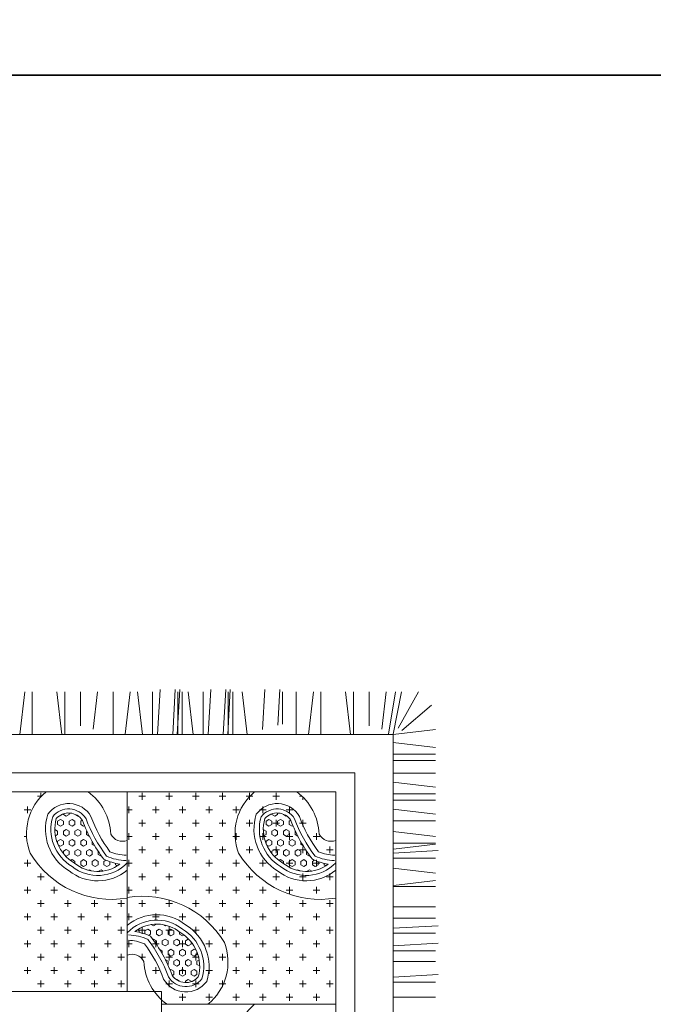
# Model space of a CAD drawing. Units: inches. Extents: x -638 to 186, y -762 to 59.
# Tile 19 of 31: x -118 to -92, y -243 to -203. Entities that reach past the tile are written whole.
import ezdxf

# ---------------------------------------------------------------- set-up
doc = ezdxf.new("R2010")
doc.units = ezdxf.units.IN
for name, color, linetype, lineweight in [('A-ANNO-DIMS', 2, 'Continuous', 18), ('furn', 8, 'Continuous', 13), ('wall', 7, 'Continuous', 35)]:
    doc.layers.add(name, color=color, linetype=linetype, lineweight=lineweight)
doc.styles.get("Standard").update_dxf_attribs({"font": 'arial.ttf'})
doc.dimstyles.new('ISO-25', dxfattribs={"dimtxt": 4, "dimasz": 4, "dimexe": 1.25, "dimexo": 0.625, "dimtad": 0, "dimlunit": 4, "dimtxsty": 'Standard', "dimcen": 2.5, "dimclrt": 256, "dimadec": 0, "dimazin": 0, "dimtfac": 1, "dimtmove": 0, "dimatfit": 3, "dimfxl": 1, "dimfxlon": 1, "dimarcsym": 0})

# ---------------------------------------------------------------- blocks, each defined once
blk = doc.blocks.new('BED-DOUBLE-WITH-NIGHTSTANDS')
for p, q in [((58.548, 11.244), (58.548, 59.951)), ((68.982, 31.914), (68.982, 1.829)), ((67.427, 30.359), (67.427, 3.384)), ((66.65, 29.582), (66.65, 4.161)), ((59.394, 16.552), (59.394, 16.825)), ((60.483, 16.552), (60.483, 16.825)), ((61.571, 16.552), (61.571, 16.825)), ((62.659, 16.552), (62.659, 16.825)), ((63.748, 16.552), (63.748, 16.825)), ((64.836, 16.726), (64.836, 16.825)), ((65.924, 16.552), (65.924, 16.825)), ((68.982, 17.003), (70.71, 16.797)), ((59.258, 16.688), (59.53, 16.688)), ((60.346, 16.688), (60.619, 16.688)), ((61.435, 16.688), (61.707, 16.688)), ((62.523, 16.688), (62.795, 16.688)), ((63.612, 16.688), (63.884, 16.688)), ((65.788, 16.688), (66.06, 16.688)), ((68.982, 16.497), (70.707, 16.497)), ((58.714, 16.144), (58.986, 16.144)), ((58.85, 16.008), (58.85, 16.28)), ((59.802, 16.144), (60.074, 16.144)), ((59.938, 16.008), (59.938, 16.28)), ((60.891, 16.144), (61.163, 16.144)), ((61.027, 16.008), (61.027, 16.28)), ((61.979, 16.144), (62.251, 16.144)), ((62.115, 16.008), (62.115, 16.28)), ((63.067, 16.144), (63.339, 16.144)), ((63.203, 16.008), (63.203, 16.28)), ((66.45, 16.144), (66.605, 16.144)), ((66.468, 16.127), (66.468, 16.28)), ((59.258, 15.6), (59.53, 15.6)), ((59.394, 15.464), (59.394, 15.736)), ((60.346, 15.6), (60.619, 15.6)), ((60.483, 15.464), (60.483, 15.736)), ((61.435, 15.6), (61.707, 15.6)), ((61.571, 15.464), (61.571, 15.736)), ((62.523, 15.6), (62.795, 15.6)), ((62.659, 15.464), (62.659, 15.736)), ((64.143, 15.233), (64.236, 15.233)), ((64.304, 15.115), (64.236, 15.233)), ((64.44, 15.351), (64.495, 15.445)), ((64.508, 15.233), (64.44, 15.351)), ((64.508, 15.233), (64.644, 15.233)), ((64.552, 15.469), (64.644, 15.469)), ((64.712, 15.351), (64.644, 15.469)), ((64.644, 15.233), (64.712, 15.351)), ((64.849, 15.115), (64.917, 15.233)), ((64.917, 15.469), (64.866, 15.556)), ((64.917, 15.469), (65.053, 15.469)), ((64.917, 15.233), (65.053, 15.233)), ((65.053, 15.469), (65.116, 15.579)), ((65.121, 15.115), (65.053, 15.233)), ((65.257, 15.351), (65.325, 15.469)), ((65.325, 15.233), (65.257, 15.351)), ((65.325, 15.469), (65.461, 15.469)), ((65.325, 15.233), (65.461, 15.233)), ((65.529, 15.351), (65.461, 15.469)), ((65.461, 15.233), (65.529, 15.351)), ((65.665, 15.115), (65.733, 15.233)), ((65.733, 15.233), (65.755, 15.233)), ((68.982, 15.294), (70.71, 15.497)), ((58.714, 15.056), (58.986, 15.056)), ((58.85, 14.92), (58.85, 15.192)), ((59.802, 15.056), (60.074, 15.056)), ((59.938, 14.92), (59.938, 15.192)), ((60.891, 15.056), (61.163, 15.056)), ((61.027, 14.92), (61.027, 15.192)), ((61.979, 15.056), (62.251, 15.056)), ((62.115, 14.92), (62.115, 15.192)), ((63.828, 14.762), (63.896, 14.88)), ((63.896, 14.88), (63.86, 14.942)), ((64.032, 15.115), (64.059, 15.161)), ((64.1, 14.997), (64.032, 15.115)), ((64.1, 14.997), (64.236, 14.997)), ((64.236, 14.997), (64.304, 15.115)), ((64.44, 14.88), (64.508, 14.997)), ((64.508, 14.762), (64.44, 14.88)), ((64.508, 14.997), (64.644, 14.997)), ((64.712, 14.88), (64.644, 14.997)), ((64.644, 14.762), (64.712, 14.88)), ((64.917, 14.997), (64.849, 15.115)), ((64.917, 14.997), (65.053, 14.997)), ((65.053, 14.997), (65.121, 15.115)), ((65.257, 14.88), (65.325, 14.997)), ((65.325, 14.762), (65.257, 14.88)), ((65.325, 14.997), (65.461, 14.997)), ((65.529, 14.88), (65.461, 14.997)), ((65.461, 14.762), (65.529, 14.88)), ((65.733, 14.997), (65.665, 15.115)), ((65.733, 14.997), (65.791, 14.997)), ((68.982, 15.174), (70.707, 15.174)), ((59.258, 14.512), (59.53, 14.512)), ((59.394, 14.376), (59.394, 14.648)), ((60.346, 14.512), (60.619, 14.512)), ((60.483, 14.376), (60.483, 14.648)), ((61.435, 14.512), (61.707, 14.512)), ((61.571, 14.376), (61.571, 14.648)), ((63.624, 14.408), (63.692, 14.526)), ((63.692, 14.291), (63.624, 14.408)), ((63.692, 14.526), (63.828, 14.526)), ((63.737, 14.762), (63.828, 14.762)), ((63.896, 14.408), (63.828, 14.526)), ((63.828, 14.291), (63.896, 14.408)), ((64.032, 14.644), (64.1, 14.762)), ((64.1, 14.526), (64.032, 14.644)), ((64.1, 14.762), (64.236, 14.762)), ((64.1, 14.526), (64.236, 14.526)), ((64.304, 14.644), (64.236, 14.762)), ((64.236, 14.526), (64.304, 14.644)), ((64.44, 14.408), (64.508, 14.526)), ((64.508, 14.291), (64.44, 14.408)), ((64.508, 14.762), (64.644, 14.762)), ((64.508, 14.526), (64.644, 14.526)), ((64.712, 14.408), (64.644, 14.526)), ((64.644, 14.291), (64.712, 14.408)), ((64.849, 14.644), (64.917, 14.762)), ((64.917, 14.526), (64.849, 14.644)), ((64.917, 14.762), (65.053, 14.762)), ((64.917, 14.526), (65.053, 14.526)), ((65.121, 14.644), (65.053, 14.762)), ((65.053, 14.526), (65.121, 14.644)), ((65.257, 14.408), (65.325, 14.526)), ((65.276, 14.375), (65.257, 14.408)), ((65.325, 14.762), (65.461, 14.762)), ((65.325, 14.526), (65.461, 14.526)), ((65.497, 14.464), (65.461, 14.526)), ((65.665, 14.644), (65.733, 14.762)), ((65.671, 14.634), (65.665, 14.644)), ((65.733, 14.762), (65.741, 14.762)), ((69.331, 14.538), (70.707, 14.538)), ((58.85, 13.832), (58.85, 14.104)), ((59.938, 13.832), (59.938, 14.104)), ((61.027, 13.832), (61.027, 14.104)), ((62.115, 13.832), (62.115, 14.104)), ((63.438, 14.086), (63.488, 14.173)), ((63.488, 14.173), (63.465, 14.213)), ((63.624, 13.937), (63.692, 14.055)), ((63.692, 14.291), (63.828, 14.291)), ((63.692, 14.055), (63.828, 14.055)), ((63.896, 13.937), (63.828, 14.055)), ((64.032, 14.173), (64.1, 14.291)), ((64.1, 14.055), (64.032, 14.173)), ((64.1, 14.291), (64.236, 14.291)), ((64.1, 14.055), (64.236, 14.055)), ((64.304, 14.173), (64.236, 14.291)), ((64.236, 14.055), (64.304, 14.173)), ((64.451, 13.955), (64.508, 14.055)), ((64.508, 14.291), (64.644, 14.291)), ((64.508, 14.055), (64.621, 14.055)), ((64.852, 14.179), (64.917, 14.291)), ((64.917, 14.291), (65.053, 14.291)), ((65.059, 14.28), (65.053, 14.291)), ((69.195, 14.023), (70.71, 13.844)), ((58.714, 13.968), (58.986, 13.968)), ((59.802, 13.968), (60.074, 13.968)), ((60.891, 13.968), (61.163, 13.968)), ((61.979, 13.968), (62.251, 13.968)), ((63.417, 13.819), (63.42, 13.819)), ((63.488, 13.701), (63.42, 13.819)), ((63.434, 13.608), (63.488, 13.701)), ((63.692, 13.819), (63.624, 13.937)), ((63.692, 13.819), (63.828, 13.819)), ((63.828, 13.819), (63.896, 13.937)), ((64.032, 13.701), (64.1, 13.819)), ((64.043, 13.682), (64.032, 13.701)), ((64.1, 13.819), (64.236, 13.819)), ((64.237, 13.818), (64.236, 13.819)), ((59.258, 13.423), (59.53, 13.423)), ((59.394, 13.287), (59.394, 13.559)), ((60.346, 13.423), (60.619, 13.423)), ((60.483, 13.287), (60.483, 13.559)), ((61.435, 13.423), (61.707, 13.423)), ((61.571, 13.287), (61.571, 13.559)), ((63.624, 13.466), (63.692, 13.584)), ((63.692, 13.348), (63.624, 13.466)), ((63.692, 13.584), (63.828, 13.584)), ((63.692, 13.348), (63.815, 13.348)), ((63.874, 13.504), (63.828, 13.584)), ((68.996, 13.214), (70.707, 13.214)), ((58.714, 12.879), (58.986, 12.879)), ((58.85, 12.743), (58.85, 13.015)), ((59.802, 12.879), (60.074, 12.879)), ((59.938, 12.743), (59.938, 13.015)), ((60.891, 12.879), (61.163, 12.879)), ((61.027, 12.743), (61.027, 13.015)), ((61.979, 12.879), (62.251, 12.879)), ((62.115, 12.743), (62.115, 13.015)), ((63.648, 13.036), (63.692, 13.112)), ((63.692, 13.112), (63.748, 13.112)), ((66.65, 12.635), (58.548, 12.635)), ((58.548, 12.635), (66.65, 12.635)), ((60.346, 12.568), (60.619, 12.568)), ((60.483, 12.432), (60.483, 12.635)), ((61.435, 12.568), (61.707, 12.568)), ((61.571, 12.432), (61.571, 12.635)), ((62.523, 12.568), (62.795, 12.568)), ((62.523, 12.568), (62.795, 12.568)), ((62.659, 12.432), (62.659, 12.635)), ((62.659, 12.432), (62.659, 12.635)), ((63.612, 12.568), (63.884, 12.568)), ((63.612, 12.568), (63.884, 12.568)), ((63.748, 12.432), (63.748, 12.635)), ((63.748, 12.432), (63.748, 12.635)), ((64.7, 12.568), (64.972, 12.568)), ((64.7, 12.568), (64.972, 12.568)), ((64.836, 12.432), (64.836, 12.635)), ((64.836, 12.432), (64.836, 12.635)), ((65.788, 12.568), (66.06, 12.568)), ((65.788, 12.568), (66.06, 12.568)), ((65.924, 12.432), (65.924, 12.635)), ((65.924, 12.432), (65.924, 12.635)), ((66.65, 12.635), (66.65, 4.161)), ((68.996, 12.723), (70.71, 12.52)), ((59.857, 12.024), (60.074, 12.024)), ((59.938, 11.888), (59.938, 12.107)), ((60.891, 12.024), (61.163, 12.024)), ((61.003, 12.157), (60.948, 12.157)), ((61.047, 12.233), (61.003, 12.157)), ((61.027, 11.888), (61.027, 12.16)), ((61.979, 12.024), (62.251, 12.024)), ((62.115, 11.888), (62.115, 12.16)), ((63.067, 12.024), (63.339, 12.024)), ((63.067, 12.024), (63.339, 12.024)), ((63.203, 11.888), (63.203, 12.16)), ((63.203, 11.888), (63.203, 12.16)), ((64.156, 12.024), (64.428, 12.024)), ((64.156, 12.024), (64.428, 12.024)), ((64.292, 11.888), (64.292, 12.16)), ((64.292, 11.888), (64.292, 12.16)), ((65.244, 12.024), (65.516, 12.024)), ((65.244, 12.024), (65.516, 12.024)), ((65.38, 11.888), (65.38, 12.16)), ((65.38, 11.888), (65.38, 12.16)), ((66.332, 12.024), (66.605, 12.024)), ((66.332, 12.024), (66.605, 12.024)), ((66.468, 11.888), (66.468, 12.16)), ((66.468, 11.888), (66.468, 12.16)), ((68.982, 12.011), (70.71, 12.214)), ((59.394, 11.344), (59.394, 11.616)), ((60.483, 11.344), (60.483, 11.616)), ((60.821, 11.766), (60.867, 11.686)), ((61.003, 11.686), (60.867, 11.686)), ((61.003, 11.921), (60.881, 11.921)), ((61.003, 11.921), (61.072, 11.804)), ((61.072, 11.804), (61.003, 11.686)), ((61.261, 11.661), (61.208, 11.568)), ((61.571, 11.344), (61.571, 11.616)), ((62.659, 11.344), (62.659, 11.616)), ((62.659, 11.344), (62.659, 11.616)), ((63.748, 11.344), (63.748, 11.616)), ((63.748, 11.344), (63.748, 11.616)), ((64.836, 11.344), (64.836, 11.616)), ((64.836, 11.344), (64.836, 11.616)), ((65.924, 11.344), (65.924, 11.616)), ((65.924, 11.344), (65.924, 11.616)), ((68.982, 11.603), (70.71, 11.603)), ((20.158, 11.244), (58.548, 11.244)), ((58.022, 4.161), (58.022, 11.244)), ((58.022, 11.244), (58.022, 4.161)), ((59.258, 11.48), (59.53, 11.48)), ((60.187, 11.215), (60.075, 11.215)), ((60.245, 11.315), (60.187, 11.215)), ((60.346, 11.48), (60.619, 11.48)), ((60.459, 11.215), (60.391, 11.097)), ((60.459, 11.451), (60.459, 11.45)), ((60.595, 11.45), (60.459, 11.45)), ((60.595, 11.215), (60.459, 11.215)), ((60.663, 11.568), (60.595, 11.45)), ((60.595, 11.215), (60.663, 11.097)), ((60.652, 11.587), (60.663, 11.568)), ((60.867, 11.45), (60.799, 11.332)), ((60.799, 11.332), (60.867, 11.215)), ((61.003, 11.45), (60.867, 11.45)), ((61.003, 11.215), (60.867, 11.215)), ((61.003, 11.45), (61.072, 11.332)), ((61.072, 11.332), (61.003, 11.215)), ((61.208, 11.568), (61.276, 11.45)), ((61.279, 11.45), (61.276, 11.45)), ((61.435, 11.48), (61.707, 11.48)), ((62.523, 11.48), (62.795, 11.48)), ((62.523, 11.48), (62.795, 11.48)), ((63.612, 11.48), (63.884, 11.48)), ((63.612, 11.48), (63.884, 11.48)), ((64.7, 11.48), (64.972, 11.48)), ((64.7, 11.48), (64.972, 11.48)), ((65.788, 11.48), (66.06, 11.48)), ((65.788, 11.48), (66.06, 11.48)), ((68.982, 11.4), (70.811, 11.298)), ((58.714, 10.936), (58.986, 10.936)), ((58.85, 10.8), (58.85, 11.072)), ((59.199, 10.806), (59.235, 10.743)), ((59.439, 10.861), (59.371, 10.743)), ((59.419, 10.895), (59.439, 10.861)), ((59.637, 10.99), (59.643, 10.979)), ((59.779, 10.979), (59.643, 10.979)), ((59.843, 11.09), (59.779, 10.979)), ((59.802, 10.936), (60.074, 10.936)), ((59.938, 10.8), (59.938, 11.072)), ((60.051, 10.979), (59.983, 10.861)), ((59.983, 10.861), (60.051, 10.743)), ((60.187, 10.979), (60.051, 10.979)), ((60.187, 10.979), (60.255, 10.861)), ((60.255, 10.861), (60.187, 10.743)), ((60.391, 11.097), (60.459, 10.979)), ((60.595, 10.979), (60.459, 10.979)), ((60.663, 11.097), (60.595, 10.979)), ((60.867, 10.979), (60.799, 10.861)), ((60.799, 10.861), (60.867, 10.743)), ((61.003, 10.979), (60.867, 10.979)), ((60.891, 10.936), (61.163, 10.936)), ((61.003, 10.979), (61.072, 10.861)), ((61.072, 10.861), (61.003, 10.743)), ((61.027, 10.8), (61.027, 11.072)), ((61.258, 11.184), (61.208, 11.097)), ((61.208, 11.097), (61.231, 11.057)), ((61.979, 10.936), (62.251, 10.936)), ((62.115, 10.8), (62.115, 11.072)), ((63.067, 10.936), (63.339, 10.936)), ((63.067, 10.936), (63.339, 10.936)), ((63.203, 10.8), (63.203, 11.072)), ((63.203, 10.8), (63.203, 11.072)), ((64.156, 10.936), (64.428, 10.936)), ((64.156, 10.936), (64.428, 10.936)), ((64.292, 10.8), (64.292, 11.072)), ((64.292, 10.8), (64.292, 11.072)), ((65.244, 10.936), (65.516, 10.936)), ((65.244, 10.936), (65.516, 10.936)), ((65.38, 10.8), (65.38, 11.072)), ((65.38, 10.8), (65.38, 11.072)), ((66.332, 10.936), (66.605, 10.936)), ((66.332, 10.936), (66.605, 10.936)), ((66.468, 10.8), (66.468, 11.072)), ((66.468, 10.8), (66.468, 11.072)), ((58.306, 10.256), (58.306, 10.528)), ((58.963, 10.508), (58.955, 10.508)), ((59.031, 10.625), (58.963, 10.508)), ((59.025, 10.636), (59.031, 10.625)), ((59.235, 10.508), (59.167, 10.39)), ((59.371, 10.743), (59.235, 10.743)), ((59.371, 10.508), (59.235, 10.508)), ((59.371, 10.508), (59.439, 10.39)), ((59.394, 10.256), (59.394, 10.528)), ((59.643, 10.743), (59.575, 10.625)), ((59.575, 10.625), (59.643, 10.508)), ((59.779, 10.743), (59.643, 10.743)), ((59.779, 10.508), (59.643, 10.508)), ((59.779, 10.743), (59.847, 10.625)), ((59.847, 10.625), (59.779, 10.508)), ((60.051, 10.508), (59.983, 10.39)), ((60.187, 10.743), (60.051, 10.743)), ((60.187, 10.508), (60.051, 10.508)), ((60.187, 10.508), (60.255, 10.39)), ((60.459, 10.743), (60.391, 10.625)), ((60.391, 10.625), (60.459, 10.508)), ((60.595, 10.743), (60.459, 10.743)), ((60.595, 10.508), (60.459, 10.508)), ((60.483, 10.256), (60.483, 10.528)), ((60.595, 10.743), (60.663, 10.625)), ((60.663, 10.625), (60.595, 10.508)), ((60.867, 10.508), (60.799, 10.39)), ((61.003, 10.743), (60.867, 10.743)), ((60.958, 10.508), (60.867, 10.508)), ((61.571, 10.256), (61.571, 10.528)), ((62.659, 10.256), (62.659, 10.528)), ((62.659, 10.256), (62.659, 10.528)), ((63.748, 10.256), (63.748, 10.528)), ((63.748, 10.256), (63.748, 10.528)), ((64.836, 10.256), (64.836, 10.528)), ((64.836, 10.256), (64.836, 10.528)), ((65.924, 10.256), (65.924, 10.528)), ((65.924, 10.256), (65.924, 10.528)), ((68.982, 10.789), (70.811, 10.687)), ((68.982, 10.606), (70.811, 10.504)), ((68.982, 10.585), (70.71, 10.585)), ((68.982, 10.402), (70.71, 10.402)), ((58.17, 10.392), (58.442, 10.392)), ((58.963, 10.272), (58.904, 10.272)), ((58.963, 10.036), (58.94, 10.036)), ((58.963, 10.272), (59.031, 10.154)), ((59.031, 10.154), (58.963, 10.036)), ((59.167, 10.39), (59.235, 10.272)), ((59.235, 10.036), (59.167, 9.919)), ((59.371, 10.272), (59.235, 10.272)), ((59.371, 10.036), (59.235, 10.036)), ((59.258, 10.392), (59.53, 10.392)), ((59.439, 10.39), (59.371, 10.272)), ((59.371, 10.036), (59.439, 9.919)), ((59.643, 10.272), (59.575, 10.154)), ((59.575, 10.154), (59.643, 10.036)), ((59.779, 10.272), (59.643, 10.272)), ((59.779, 10.036), (59.643, 10.036)), ((59.779, 10.272), (59.847, 10.154)), ((59.847, 10.154), (59.779, 10.036)), ((59.983, 10.39), (60.051, 10.272)), ((60.051, 10.036), (59.983, 9.919)), ((60.187, 10.272), (60.051, 10.272)), ((60.187, 10.036), (60.051, 10.036)), ((60.255, 10.39), (60.187, 10.272)), ((60.187, 10.036), (60.255, 9.919)), ((60.346, 10.392), (60.619, 10.392)), ((60.459, 10.272), (60.391, 10.154)), ((60.391, 10.154), (60.459, 10.036)), ((60.595, 10.272), (60.459, 10.272)), ((60.553, 10.036), (60.459, 10.036)), ((60.595, 10.272), (60.663, 10.154)), ((60.663, 10.154), (60.637, 10.108)), ((60.799, 10.39), (60.836, 10.327)), ((61.435, 10.392), (61.707, 10.392)), ((62.523, 10.392), (62.795, 10.392)), ((62.523, 10.392), (62.795, 10.392)), ((63.612, 10.392), (63.884, 10.392)), ((63.612, 10.392), (63.884, 10.392)), ((64.7, 10.392), (64.972, 10.392)), ((64.7, 10.392), (64.972, 10.392)), ((65.788, 10.392), (66.06, 10.392)), ((65.788, 10.392), (66.06, 10.392)), ((68.982, 9.957), (70.71, 10.161)), ((58.714, 9.847), (58.986, 9.847)), ((58.85, 9.711), (58.85, 9.983)), ((59.167, 9.919), (59.235, 9.801)), ((59.371, 9.801), (59.235, 9.801)), ((59.439, 9.919), (59.371, 9.801)), ((59.643, 9.801), (59.58, 9.691)), ((59.779, 9.801), (59.643, 9.801)), ((59.779, 9.801), (59.83, 9.713)), ((59.802, 9.847), (60.074, 9.847)), ((59.938, 9.711), (59.938, 9.983)), ((59.983, 9.919), (60.051, 9.801)), ((60.144, 9.801), (60.051, 9.801)), ((60.255, 9.919), (60.201, 9.825)), ((60.891, 9.847), (61.163, 9.847)), ((61.027, 9.711), (61.027, 9.983)), ((61.979, 9.847), (62.251, 9.847)), ((61.979, 9.847), (62.251, 9.847)), ((62.115, 9.711), (62.115, 9.983)), ((62.115, 9.711), (62.115, 9.983)), ((63.067, 9.847), (63.339, 9.847)), ((63.067, 9.847), (63.339, 9.847)), ((63.203, 9.711), (63.203, 9.983)), ((63.203, 9.711), (63.203, 9.983)), ((64.156, 9.847), (64.428, 9.847)), ((64.156, 9.847), (64.428, 9.847)), ((64.292, 9.711), (64.292, 9.983)), ((64.292, 9.711), (64.292, 9.983)), ((65.244, 9.847), (65.516, 9.847)), ((65.244, 9.847), (65.516, 9.847)), ((65.38, 9.711), (65.38, 9.983)), ((65.38, 9.711), (65.38, 9.983)), ((66.332, 9.847), (66.605, 9.847)), ((66.332, 9.847), (66.605, 9.847)), ((66.468, 9.711), (66.468, 9.983)), ((66.468, 9.711), (66.468, 9.983)), ((58.17, 9.303), (58.442, 9.303)), ((58.306, 9.167), (58.306, 9.439)), ((59.258, 9.303), (59.53, 9.303)), ((59.394, 9.167), (59.394, 9.439)), ((60.346, 9.303), (60.619, 9.303)), ((60.483, 9.167), (60.483, 9.439)), ((61.435, 9.303), (61.707, 9.303)), ((61.435, 9.303), (61.707, 9.303)), ((61.571, 9.167), (61.571, 9.439)), ((61.571, 9.167), (61.571, 9.439)), ((62.523, 9.303), (62.795, 9.303)), ((62.523, 9.303), (62.795, 9.303)), ((62.659, 9.167), (62.659, 9.439)), ((62.659, 9.167), (62.659, 9.439)), ((63.612, 9.303), (63.884, 9.303)), ((63.612, 9.303), (63.884, 9.303)), ((63.748, 9.167), (63.748, 9.439)), ((63.748, 9.167), (63.748, 9.439)), ((64.7, 9.303), (64.972, 9.303)), ((64.7, 9.303), (64.972, 9.303)), ((64.836, 9.167), (64.836, 9.439)), ((64.836, 9.167), (64.836, 9.439)), ((65.788, 9.303), (66.06, 9.303)), ((65.788, 9.303), (66.06, 9.303)), ((65.924, 9.167), (65.924, 9.439)), ((65.924, 9.167), (65.924, 9.439)), ((68.982, 9.55), (70.71, 9.55)), ((68.982, 9.347), (70.811, 9.245)), ((58.85, 8.623), (58.85, 8.895)), ((59.938, 8.623), (59.938, 8.895)), ((61.027, 8.623), (61.027, 8.895)), ((61.027, 8.623), (61.027, 8.895)), ((62.115, 8.623), (62.115, 8.895)), ((62.115, 8.623), (62.115, 8.895)), ((63.203, 8.623), (63.203, 8.895)), ((63.203, 8.623), (63.203, 8.895)), ((64.292, 8.623), (64.292, 8.895)), ((64.292, 8.623), (64.292, 8.895)), ((65.38, 8.623), (65.38, 8.895)), ((65.38, 8.623), (65.38, 8.895)), ((66.468, 8.623), (66.468, 8.895)), ((66.468, 8.623), (66.468, 8.895)), ((58.714, 8.759), (58.783, 8.759)), ((58.714, 8.759), (58.986, 8.759)), ((58.85, 8.623), (58.85, 8.728)), ((59.802, 8.759), (60.074, 8.759)), ((60.891, 8.759), (61.163, 8.759)), ((60.891, 8.759), (61.163, 8.759)), ((61.979, 8.759), (62.251, 8.759)), ((61.979, 8.759), (62.251, 8.759)), ((63.067, 8.759), (63.339, 8.759)), ((63.067, 8.759), (63.339, 8.759)), ((64.156, 8.759), (64.428, 8.759)), ((64.156, 8.759), (64.428, 8.759)), ((65.244, 8.759), (65.516, 8.759)), ((65.244, 8.759), (65.516, 8.759)), ((66.332, 8.759), (66.605, 8.759)), ((66.332, 8.759), (66.605, 8.759)), ((68.982, 8.736), (70.811, 8.634)), ((68.982, 8.553), (70.811, 8.451)), ((68.982, 8.532), (70.71, 8.532)), ((58.17, 8.215), (58.442, 8.215)), ((58.17, 8.215), (58.442, 8.215)), ((58.306, 8.079), (58.306, 8.351)), ((58.306, 8.079), (58.306, 8.351)), ((59.258, 8.215), (59.53, 8.215)), ((59.258, 8.215), (59.53, 8.215)), ((59.394, 8.079), (59.394, 8.351)), ((59.394, 8.079), (59.394, 8.351)), ((60.346, 8.215), (60.619, 8.215)), ((60.346, 8.215), (60.619, 8.215)), ((60.483, 8.079), (60.483, 8.351)), ((60.483, 8.079), (60.483, 8.351)), ((61.435, 8.215), (61.707, 8.215)), ((61.435, 8.215), (61.707, 8.215)), ((61.571, 8.079), (61.571, 8.351)), ((61.571, 8.079), (61.571, 8.351)), ((62.523, 8.215), (62.795, 8.215)), ((62.523, 8.215), (62.795, 8.215)), ((62.659, 8.079), (62.659, 8.351)), ((62.659, 8.079), (62.659, 8.351)), ((63.612, 8.215), (63.884, 8.215)), ((63.612, 8.215), (63.884, 8.215)), ((63.748, 8.079), (63.748, 8.351)), ((63.748, 8.079), (63.748, 8.351)), ((64.7, 8.215), (64.972, 8.215)), ((64.836, 8.253), (64.836, 8.351)), ((64.836, 8.079), (64.836, 8.351)), ((65.788, 8.215), (66.06, 8.215)), ((65.788, 8.215), (66.06, 8.215)), ((65.924, 8.079), (65.924, 8.351)), ((65.924, 8.079), (65.924, 8.351)), ((68.982, 8.349), (70.71, 8.349)), ((58.714, 7.671), (58.986, 7.671)), ((58.714, 7.671), (58.986, 7.671)), ((58.85, 7.535), (58.85, 7.807)), ((58.85, 7.535), (58.85, 7.807)), ((59.802, 7.671), (60.074, 7.671)), ((59.802, 7.671), (60.074, 7.671)), ((59.938, 7.535), (59.938, 7.807)), ((59.938, 7.535), (59.938, 7.807)), ((60.891, 7.671), (61.163, 7.671)), ((60.891, 7.671), (61.163, 7.671)), ((61.027, 7.535), (61.027, 7.807)), ((61.027, 7.535), (61.027, 7.807)), ((61.979, 7.671), (62.251, 7.671)), ((61.979, 7.671), (62.251, 7.671)), ((62.115, 7.535), (62.115, 7.807)), ((62.115, 7.535), (62.115, 7.807)), ((63.067, 7.671), (63.339, 7.671)), ((63.067, 7.671), (63.339, 7.671)), ((63.203, 7.535), (63.203, 7.807)), ((63.203, 7.535), (63.203, 7.807)), ((64.156, 7.671), (64.428, 7.671)), ((64.292, 7.535), (64.292, 7.807)), ((65.244, 7.671), (65.516, 7.671)), ((65.38, 7.535), (65.38, 7.807)), ((66.332, 7.671), (66.605, 7.671)), ((66.45, 7.671), (66.605, 7.671)), ((66.468, 7.653), (66.468, 7.807)), ((66.468, 7.535), (66.468, 7.807)), ((68.982, 7.757), (70.71, 7.961)), ((58.306, 6.99), (58.306, 7.263)), ((58.306, 6.99), (58.306, 7.263)), ((59.394, 6.99), (59.394, 7.263)), ((59.394, 6.99), (59.394, 7.263)), ((60.483, 6.99), (60.483, 7.263)), ((60.483, 6.99), (60.483, 7.263)), ((61.571, 6.99), (61.571, 7.263)), ((61.571, 6.99), (61.571, 7.263)), ((62.659, 6.99), (62.659, 7.263)), ((62.659, 6.99), (62.659, 7.263)), ((63.748, 6.99), (63.748, 7.263)), ((64.836, 6.99), (64.836, 7.263)), ((65.924, 6.99), (65.924, 7.263)), ((58.17, 7.127), (58.442, 7.127)), ((58.17, 7.127), (58.442, 7.127)), ((59.258, 7.127), (59.53, 7.127)), ((59.258, 7.127), (59.53, 7.127)), ((60.346, 7.127), (60.619, 7.127)), ((60.346, 7.127), (60.619, 7.127)), ((61.435, 7.127), (61.707, 7.127)), ((61.435, 7.127), (61.707, 7.127)), ((62.523, 7.127), (62.795, 7.127)), ((62.523, 7.127), (62.795, 7.127)), ((63.612, 7.127), (63.884, 7.127)), ((64.44, 6.877), (64.495, 6.971)), ((64.508, 6.76), (64.44, 6.877)), ((64.552, 6.995), (64.644, 6.995)), ((64.712, 6.877), (64.644, 6.995)), ((64.644, 6.76), (64.712, 6.877)), ((64.7, 7.127), (64.972, 7.127)), ((64.917, 6.995), (64.866, 7.082)), ((64.917, 6.995), (65.053, 6.995)), ((65.053, 6.995), (65.116, 7.105)), ((65.257, 6.877), (65.325, 6.995)), ((65.325, 6.76), (65.257, 6.877)), ((65.325, 6.995), (65.461, 6.995)), ((65.529, 6.877), (65.461, 6.995)), ((65.461, 6.76), (65.529, 6.877)), ((65.788, 7.127), (66.06, 7.127)), ((69.184, 7.135), (70.811, 7.044)), ((58.714, 6.582), (58.986, 6.582)), ((58.714, 6.582), (58.986, 6.582)), ((58.85, 6.446), (58.85, 6.718)), ((58.85, 6.446), (58.85, 6.718)), ((59.802, 6.582), (60.074, 6.582)), ((59.802, 6.582), (60.074, 6.582)), ((59.938, 6.446), (59.938, 6.718)), ((59.938, 6.446), (59.938, 6.718)), ((60.891, 6.582), (61.163, 6.582)), ((60.891, 6.582), (61.163, 6.582)), ((61.027, 6.446), (61.027, 6.718)), ((61.027, 6.446), (61.027, 6.718)), ((61.979, 6.582), (62.251, 6.582)), ((61.979, 6.582), (62.251, 6.582)), ((62.115, 6.446), (62.115, 6.718)), ((62.115, 6.446), (62.115, 6.718)), ((63.067, 6.582), (63.339, 6.582)), ((63.203, 6.446), (63.203, 6.718)), ((63.828, 6.288), (63.896, 6.406)), ((63.896, 6.406), (63.86, 6.469)), ((64.032, 6.642), (64.059, 6.688)), ((64.1, 6.524), (64.032, 6.642)), ((64.1, 6.524), (64.236, 6.524)), ((64.143, 6.76), (64.236, 6.76)), ((64.156, 6.582), (64.428, 6.582)), ((64.304, 6.642), (64.236, 6.76)), ((64.236, 6.524), (64.304, 6.642)), ((64.292, 6.446), (64.292, 6.718)), ((64.44, 6.406), (64.508, 6.524)), ((64.508, 6.288), (64.44, 6.406)), ((64.508, 6.76), (64.644, 6.76)), ((64.508, 6.524), (64.644, 6.524)), ((64.712, 6.406), (64.644, 6.524)), ((64.644, 6.288), (64.712, 6.406)), ((64.849, 6.642), (64.917, 6.76)), ((64.917, 6.524), (64.849, 6.642)), ((64.917, 6.76), (65.053, 6.76)), ((64.917, 6.524), (65.053, 6.524)), ((65.121, 6.642), (65.053, 6.76)), ((65.053, 6.524), (65.121, 6.642)), ((65.244, 6.582), (65.516, 6.582)), ((65.257, 6.406), (65.325, 6.524)), ((65.325, 6.288), (65.257, 6.406)), ((65.325, 6.76), (65.461, 6.76)), ((65.325, 6.524), (65.461, 6.524)), ((65.38, 6.446), (65.38, 6.718)), ((65.529, 6.406), (65.461, 6.524)), ((65.461, 6.288), (65.529, 6.406)), ((65.665, 6.642), (65.733, 6.76)), ((65.733, 6.524), (65.665, 6.642)), ((65.733, 6.76), (65.755, 6.76)), ((65.733, 6.524), (65.791, 6.524)), ((66.332, 6.582), (66.605, 6.582)), ((66.468, 6.446), (66.468, 6.718)), ((69.357, 6.514), (70.811, 6.433)), ((58.17, 6.038), (58.442, 6.038)), ((58.17, 6.038), (58.442, 6.038)), ((58.306, 5.902), (58.306, 6.174)), ((58.306, 5.902), (58.306, 6.174)), ((59.258, 6.038), (59.53, 6.038)), ((59.258, 6.038), (59.53, 6.038)), ((59.394, 5.902), (59.394, 6.174)), ((59.394, 5.902), (59.394, 6.174)), ((60.346, 6.038), (60.619, 6.038)), ((60.346, 6.038), (60.619, 6.038)), ((60.483, 5.902), (60.483, 6.174)), ((60.483, 5.902), (60.483, 6.174)), ((61.435, 6.038), (61.707, 6.038)), ((61.435, 6.038), (61.707, 6.038)), ((61.571, 5.902), (61.571, 6.174)), ((61.571, 5.902), (61.571, 6.174)), ((62.523, 6.038), (62.795, 6.038)), ((62.659, 5.902), (62.659, 6.174)), ((63.612, 6.038), (63.884, 6.038)), ((63.624, 5.935), (63.692, 6.053)), ((63.692, 6.053), (63.828, 6.053)), ((63.737, 6.288), (63.828, 6.288)), ((63.748, 5.902), (63.748, 6.174)), ((63.896, 5.935), (63.828, 6.053)), ((64.032, 6.17), (64.1, 6.288)), ((64.1, 6.053), (64.032, 6.17)), ((64.1, 6.288), (64.236, 6.288)), ((64.1, 6.053), (64.236, 6.053)), ((64.304, 6.17), (64.236, 6.288)), ((64.236, 6.053), (64.304, 6.17)), ((64.44, 5.935), (64.508, 6.053)), ((64.508, 6.288), (64.644, 6.288)), ((64.508, 6.053), (64.644, 6.053)), ((64.712, 5.935), (64.644, 6.053)), ((64.7, 6.038), (64.972, 6.038)), ((64.836, 5.902), (64.836, 6.174)), ((64.849, 6.17), (64.917, 6.288)), ((64.917, 6.053), (64.849, 6.17)), ((64.917, 6.288), (65.053, 6.288)), ((64.917, 6.053), (65.053, 6.053)), ((65.121, 6.17), (65.053, 6.288)), ((65.053, 6.053), (65.121, 6.17)), ((65.257, 5.935), (65.325, 6.053)), ((65.325, 6.288), (65.461, 6.288)), ((65.325, 6.053), (65.461, 6.053)), ((65.497, 5.99), (65.461, 6.053)), ((65.665, 6.17), (65.733, 6.288)), ((65.671, 6.16), (65.665, 6.17)), ((65.733, 6.288), (65.741, 6.288)), ((65.788, 6.038), (66.06, 6.038)), ((65.924, 5.902), (65.924, 6.174)), ((69.393, 6.332), (70.71, 6.332)), ((58.85, 5.358), (58.85, 5.63)), ((58.85, 5.358), (58.85, 5.63)), ((59.938, 5.358), (59.938, 5.63)), ((59.938, 5.358), (59.938, 5.63)), ((61.027, 5.358), (61.027, 5.63)), ((61.027, 5.358), (61.027, 5.63)), ((62.115, 5.358), (62.115, 5.63)), ((62.115, 5.358), (62.115, 5.63)), ((63.203, 5.358), (63.203, 5.63)), ((63.438, 5.612), (63.488, 5.699)), ((63.488, 5.699), (63.465, 5.739)), ((63.692, 5.817), (63.624, 5.935)), ((63.692, 5.817), (63.828, 5.817)), ((63.828, 5.817), (63.896, 5.935)), ((64.032, 5.699), (64.1, 5.817)), ((64.1, 5.581), (64.032, 5.699)), ((64.1, 5.817), (64.236, 5.817)), ((64.304, 5.699), (64.236, 5.817)), ((64.236, 5.581), (64.304, 5.699)), ((64.292, 5.358), (64.292, 5.63)), ((64.508, 5.817), (64.44, 5.935)), ((64.508, 5.817), (64.644, 5.817)), ((64.644, 5.817), (64.712, 5.935)), ((64.852, 5.706), (64.917, 5.817)), ((64.917, 5.817), (65.053, 5.817)), ((65.059, 5.806), (65.053, 5.817)), ((65.276, 5.901), (65.257, 5.935)), ((65.38, 5.358), (65.38, 5.63)), ((66.468, 5.533), (66.468, 5.63)), ((68.982, 5.764), (70.707, 5.764)), ((58.714, 5.494), (58.986, 5.494)), ((58.714, 5.494), (58.986, 5.494)), ((59.802, 5.494), (60.074, 5.494)), ((59.802, 5.494), (60.074, 5.494)), ((60.891, 5.494), (61.163, 5.494)), ((60.891, 5.494), (61.163, 5.494)), ((61.979, 5.494), (62.251, 5.494)), ((61.979, 5.494), (62.251, 5.494)), ((63.067, 5.494), (63.339, 5.494)), ((63.417, 5.346), (63.42, 5.346)), ((63.488, 5.228), (63.42, 5.346)), ((63.434, 5.135), (63.488, 5.228)), ((63.624, 5.464), (63.692, 5.581)), ((63.692, 5.346), (63.624, 5.464)), ((63.692, 5.581), (63.828, 5.581)), ((63.692, 5.346), (63.828, 5.346)), ((63.896, 5.464), (63.828, 5.581)), ((63.828, 5.346), (63.896, 5.464)), ((64.032, 5.228), (64.1, 5.346)), ((64.043, 5.209), (64.032, 5.228)), ((64.1, 5.581), (64.236, 5.581)), ((64.1, 5.346), (64.236, 5.346)), ((64.156, 5.494), (64.428, 5.494)), ((64.237, 5.344), (64.236, 5.346)), ((64.451, 5.481), (64.508, 5.581)), ((64.508, 5.581), (64.621, 5.581)), ((65.244, 5.494), (65.516, 5.494)), ((66.332, 5.494), (66.43, 5.494)), ((68.982, 5.274), (70.71, 5.069)), ((58.17, 4.95), (58.442, 4.95)), ((58.17, 4.95), (58.442, 4.95)), ((58.306, 4.814), (58.306, 5.086)), ((58.306, 4.814), (58.306, 5.086)), ((59.258, 4.95), (59.53, 4.95)), ((59.258, 4.95), (59.53, 4.95)), ((59.394, 4.814), (59.394, 5.086)), ((59.394, 4.814), (59.394, 5.086)), ((60.346, 4.95), (60.619, 4.95)), ((60.346, 4.95), (60.619, 4.95)), ((60.483, 4.814), (60.483, 5.086)), ((60.483, 4.814), (60.483, 5.086)), ((61.435, 4.95), (61.707, 4.95)), ((61.435, 4.95), (61.707, 4.95)), ((61.571, 4.814), (61.571, 5.086)), ((61.571, 4.814), (61.571, 5.086)), ((62.523, 4.95), (62.795, 4.95)), ((62.659, 4.814), (62.659, 5.086)), ((63.612, 4.95), (63.884, 4.95)), ((63.624, 4.992), (63.692, 5.11)), ((63.692, 4.874), (63.624, 4.992)), ((63.692, 5.11), (63.828, 5.11)), ((63.692, 4.874), (63.815, 4.874)), ((63.748, 4.814), (63.748, 5.086)), ((63.874, 5.03), (63.828, 5.11)), ((64.7, 4.95), (64.972, 4.95)), ((64.836, 4.814), (64.836, 5.086)), ((58.714, 4.406), (58.986, 4.406)), ((58.714, 4.406), (58.986, 4.406)), ((58.85, 4.27), (58.85, 4.542)), ((58.85, 4.27), (58.85, 4.542)), ((59.802, 4.406), (60.074, 4.406)), ((59.802, 4.406), (60.074, 4.406)), ((59.938, 4.27), (59.938, 4.542)), ((59.938, 4.27), (59.938, 4.542)), ((60.891, 4.406), (61.163, 4.406)), ((60.891, 4.406), (61.163, 4.406)), ((61.027, 4.27), (61.027, 4.542)), ((61.027, 4.27), (61.027, 4.542)), ((61.979, 4.406), (62.251, 4.406)), ((61.979, 4.406), (62.251, 4.406)), ((62.115, 4.27), (62.115, 4.542)), ((62.115, 4.27), (62.115, 4.542)), ((63.067, 4.406), (63.339, 4.406)), ((63.203, 4.27), (63.203, 4.542)), ((63.648, 4.563), (63.692, 4.639)), ((63.692, 4.639), (63.748, 4.639)), ((64.156, 4.406), (64.428, 4.406)), ((64.292, 4.27), (64.292, 4.542)), ((68.982, 4.769), (70.707, 4.769)), ((66.65, 4.161), (40.767, 4.161)), ((66.65, 4.161), (58.022, 4.161)), ((68.982, 3.565), (70.71, 3.769)), ((67.427, 3.384), (39.99, 3.384)), ((68.982, 3.446), (70.707, 3.446)), ((69.331, 2.81), (70.707, 2.81)), ((68.996, 2.022), (70.707, 1.732)), ((69.195, 2.295), (70.71, 2.115)), ((68.982, 1.829), (38.435, 1.829)), ((58.312, 1.829), (58.312, 0.102)), ((58.923, 1.829), (58.923, 0.102)), ((59.126, 1.829), (59.228, 0)), ((59.755, 1.815), (59.755, 0.105)), ((60.193, 1.829), (60.193, 0.102)), ((60.397, 1.829), (60.499, 0)), ((60.906, 1.829), (60.906, 0.102)), ((61.11, 1.829), (61.212, 0)), ((61.517, 1.829), (61.517, 0.102)), ((61.977, 1.829), (61.977, 0.102)), ((62.81, 1.815), (62.81, 0.105)), ((62.841, 1.815), (63.044, 0.102)), ((63.554, 1.829), (63.35, 0.102)), ((63.961, 1.829), (63.961, 0.102)), ((64.165, 1.829), (64.266, 0)), ((64.327, 1.815), (64.531, 0.102)), ((64.572, 1.829), (64.572, 0.102)), ((65.04, 1.829), (64.836, 0.102)), ((65.476, 1.829), (65.476, 0.102)), ((65.944, 1.829), (65.741, 0.102)), ((66.309, 1.815), (66.309, 0.105)), ((66.573, 1.829), (66.573, 0.102)), ((67.041, 1.829), (66.838, 0.102)), ((67.406, 1.815), (67.406, 0.105)), ((67.922, 1.815), (67.922, 0.105)), ((68.186, 1.829), (68.186, 0.102)), ((68.654, 1.829), (68.45, 0.102)), ((68.982, 1.829), (69.186, 0.102)), ((68.996, 1.829), (70.707, 1.486)), ((69.232, 1.631), (70.71, 0.792)), ((69.142, 1.47), (70.169, 0.275))]:
    blk.add_line(p, q)
for centre, radius, start, end in [((66.165, 13.26), 3.88, 121.1125, 189.2666), ((64.955, 14.528), 2.202, 39.6653, 111.1583), ((65.133, 13.987), 1.972, 72.055, 149.019), ((65.133, 13.987), 1.754, 73.2189, 149.4808), ((65.126, 15.016), 0.829, 301.6232, 51.6957), ((65.126, 15.016), 1.047, 300.344, 54.0192), ((65.133, 13.987), 1.591, 74.3738, 149.9117), ((65.126, 15.016), 0.666, 302.9498, 49.099), ((64.914, 13.836), 1.878, 141.5973, 219.7611), ((64.914, 13.836), 1.66, 141.1107, 226.3387), ((64.914, 13.836), 1.497, 140.6541, 216.833), ((67.553, 8.875), 5.952, 110.2997, 127.7385), ((67.553, 8.875), 5.789, 110.1318, 127.346), ((67.553, 8.875), 5.571, 109.9219, 126.7677), ((64.84, 15.553), 2.246, 272.4675, 323.7193), ((65.96, 12.613), 2.268, 154.7059, 171.7535), ((65.96, 12.613), 2.104, 155.7609, 178.0373), ((65.96, 12.613), 1.887, 157.4091, 178.0373), ((65.181, 12.828), 0.54, 117.0088, 201.0409), ((59.514, 12.441), 0.54, 297.0088, 21.0409), ((58.736, 12.656), 1.887, 337.4091, 358.0373), ((58.53, 12.01), 3.88, 301.1125, 9.2666), ((58.736, 12.656), 2.104, 335.7609, 358.0373), ((59.782, 11.434), 1.66, 321.1107, 46.3387), ((59.782, 11.434), 1.878, 321.5973, 39.7611), ((58.736, 12.656), 2.268, 334.7059, 351.7535), ((59.782, 11.434), 1.497, 320.6541, 36.833), ((59.856, 9.717), 2.246, 92.4675, 144.7393), ((57.143, 16.395), 5.571, 289.9219, 306.7677), ((57.143, 16.395), 5.789, 290.1318, 307.346), ((57.143, 16.395), 5.952, 290.2997, 307.7385), ((59.57, 10.253), 1.047, 120.344, 234.0192), ((59.57, 10.253), 0.829, 121.6232, 231.6957), ((59.57, 10.253), 0.666, 122.9498, 229.099), ((59.563, 11.282), 1.591, 254.3738, 329.9117), ((59.563, 11.282), 1.972, 252.055, 329.019), ((59.563, 11.282), 1.754, 253.2189, 329.4808), ((59.74, 10.742), 2.202, 218.7027, 291.1583), ((56.328, 6.054), 2.202, 39.6653, 111.1583), ((66.165, 4.786), 3.88, 121.1125, 189.2666), ((64.955, 6.054), 2.202, 39.6653, 111.1583), ((65.133, 5.514), 1.972, 72.055, 149.019), ((65.133, 5.514), 1.754, 73.2189, 149.4808), ((65.126, 6.543), 1.047, 300.344, 54.0192), ((65.133, 5.514), 1.591, 74.3738, 149.9117), ((65.126, 6.543), 0.666, 302.9498, 49.099), ((65.126, 6.543), 0.829, 301.6232, 51.6957), ((64.914, 5.362), 1.878, 141.5973, 219.7611), ((64.914, 5.362), 1.66, 141.1107, 226.3387), ((64.914, 5.362), 1.497, 140.6541, 216.833), ((67.553, 0.401), 5.952, 110.2997, 127.7385), ((67.553, 0.401), 5.789, 110.1318, 127.346), ((67.553, 0.401), 5.571, 109.9219, 126.7677), ((64.84, 7.079), 2.246, 272.4675, 323.7193), ((65.96, 4.14), 2.268, 154.7059, 171.7535), ((65.96, 4.14), 2.104, 155.7609, 178.0373), ((65.96, 4.14), 1.887, 157.4091, 178.0373), ((65.181, 4.355), 0.54, 117.0088, 201.0409)]:
    blk.add_arc(centre, radius, start, end)
blk = doc.blocks.new('*D37')
at = {"layer": 'A-ANNO-DIMS', "color": 0, "lineweight": -2, "transparency": 16777216}
for p, q in [((182.663, -232.533), (184.913, -232.533)), ((183.663, -236.533), (183.663, -250.511)), ((183.663, -276.533), (183.663, -262.555)), ((182.663, -280.533), (184.913, -280.533))]:
    blk.add_line(p, q, dxfattribs=at)
at = {"layer": 'A-ANNO-DIMS', "color": 0, "lineweight": 30, "transparency": 16777216}
for points in [[(182.997, -236.533), (184.33, -236.533), (183.663, -232.533)], [(182.997, -276.533), (184.33, -276.533), (183.663, -280.533)]]:
    blk.add_solid(points, dxfattribs=at)
at = {"layer": 'Defpoints', "color": 0, "lineweight": 30, "transparency": 16777216}
for p in [(-404.526, -232.533), (-404.526, -280.533), (183.663, -280.533)]:
    blk.add_point(p, dxfattribs=at)
at = {"layer": 'A-ANNO-DIMS', "transparency": 16777216, "insert": (183.663, -256.533), "char_height": 4, "attachment_point": 5, "rotation": 90}
blk.add_mtext('4\'-0"', dxfattribs=at)
blk = doc.blocks.new('*D56')
at = {"layer": 'A-ANNO-DIMS', "color": 0, "lineweight": -2, "transparency": 16777216}
for p, q in [((-165.026, 52.017), (-165.026, 54.267)), ((-100.526, 52.017), (-100.526, 54.267)), ((-161.026, 53.017), (-143.378, 53.017)), ((-104.526, 53.017), (-122.174, 53.017))]:
    blk.add_line(p, q, dxfattribs=at)
at = {"layer": 'A-ANNO-DIMS', "color": 0, "lineweight": 30, "transparency": 16777216}
for points in [[(-161.026, 53.684), (-161.026, 52.35), (-165.026, 53.017)], [(-104.526, 53.684), (-104.526, 52.35), (-100.526, 53.017)]]:
    blk.add_solid(points, dxfattribs=at)
at = {"layer": 'Defpoints', "color": 0, "lineweight": 30, "transparency": 16777216}
for p in [(-100.526, 53.017), (-165.026, -408.033), (-100.526, -408.033)]:
    blk.add_point(p, dxfattribs=at)
at = {"layer": 'A-ANNO-DIMS', "transparency": 16777216, "insert": (-132.776, 53.017), "char_height": 4, "attachment_point": 5}
blk.add_mtext('5\'-4 1/2"', dxfattribs=at)

msp = doc.modelspace()

# ---------------------------------------------------------------- linework, layer by layer
at = {"layer": 'wall'}
msp.add_line((-160.526, -205.533), (1.474, -205.533), dxfattribs=at)

# ---------------------------------------------------------------- block references
at = {"layer": 'furn', "rotation": 90.00000000000006}
msp.add_blockref('BED-DOUBLE-WITH-NIGHTSTANDS', (-100.575, -301.287), dxfattribs=at)

# ---------------------------------------------------------------- dimensions: what is measured, and where the dimension line sits
at = {"layer": 'A-ANNO-DIMS'}
dim = msp.add_linear_dim(base=(-100.526, 53.017), p1=(-165.026, -408.033), p2=(-100.526, -408.033), dimstyle='ISO-25', override={"dimdec": 1, "dimlfac": 1, "dimrnd": 0, "dimzin": 1, "dimdsep": 46, "dimlunit": 4, "dimfrac": 2}, dxfattribs=at)
dim.commit()
dim.dimension.update_dxf_attribs({"geometry": '*D56', "text_midpoint": (-132.776, 53.017)})
dim = msp.add_linear_dim(base=(183.663, -280.533), p1=(-404.526, -232.533), p2=(-404.526, -280.533), angle=90, dimstyle='ISO-25', override={"dimdec": 1, "dimlfac": 1, "dimrnd": 0, "dimzin": 1, "dimdsep": 46, "dimlunit": 4, "dimfrac": 2}, dxfattribs=at)
dim.commit()
dim.dimension.update_dxf_attribs({"geometry": '*D37', "text_midpoint": (183.663, -256.533)})

doc.saveas('drawing.dxf')
